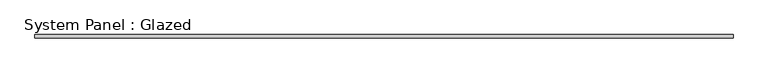
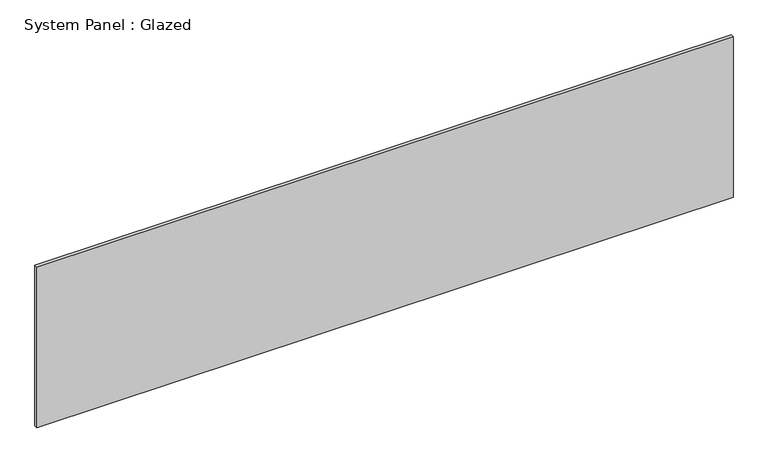
"""IFC4 building model written with IfcOpenShell, lengths in millimetres: plate geometry, System Panel : Glazed."""

from ifc_helpers import new_model, si_unit, origin, origin_with_axes, place, context, project, spatial, polyline, outline, extrude, source, transform, mapped, element, save


def system_panel_glazed_0f7bc74d(model_context):
    return source(origin(), model_context, "Body", "SweptSolid", [
        extrude(outline(polyline([(2506.7653238, 19.05), (-2506.7653238, 19.05), (-2506.7653238, 44.45), (2506.7653238, 44.45), (2506.7653238, 19.05)])), origin_with_axes(), (0.0, 0.0, 1.0), 1219.352721),
    ])


if __name__ == "__main__":
    model = new_model("IFC4")
    model_context = context("Model", 3, world=origin())
    ifc_project = project(units=[si_unit("LENGTHUNIT", "METRE", prefix="MILLI")], contexts=[model_context])
    site = spatial("IfcSite", under=ifc_project)
    building = spatial("IfcBuilding", under=site)
    placement = place(None, origin())
    system_panel_glazed_shape = system_panel_glazed_0f7bc74d(model_context)
    element("IfcPlate", 1, ObjectType="System Panel : Glazed", at=placement, inside=building, context=model_context, shape_type="MappedRepresentation", body=[
        mapped(system_panel_glazed_shape, transform((0.0, 0.0, 0.0), x_axis=(1.0, 0.0, 0.0), y_axis=(0.0, 1.0, 0.0), z_axis=(0.0, 0.0, 1.0))),
    ])
    save(model, "model.ifc")

# Revit data of these elements
# Type "System Panel : Glazed"
#   Construction Type Id = "GSP4R"
#   Analytic Construction = "1/8 in Pilkington single glazing"
#   Visual Light Transmittance = 0.9
#   Solar Heat Gain Coefficient = 0.86
#   Heat Transfer Coefficient (U) = 1.18115 BTU/(h·ft²·°F)
#   Define Thermal Properties by = 1
# Element 1 (IfcPlate, "System Panel : Glazed")
#   Materials on its faces: "Glass"
# Materials
#   "Glass": class "Glass", colour RGB 0 128 192, transparency 0.75, Description = "Soda Lime Glass", Cost = 0
